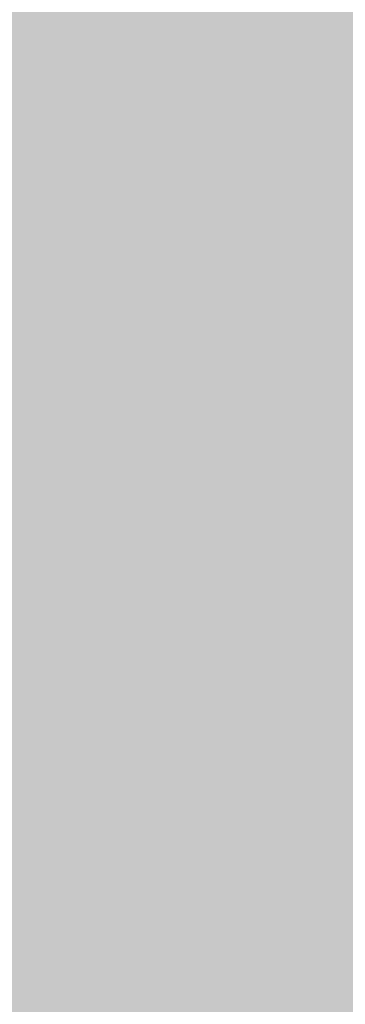
# Model space of a CAD drawing. Units: millimetres. Extents: x 0 to 2267, y 0 to 1823.
# Tile 42 of 256: x 1593.4507 to 1593.5605, y 1226.3857 to 1226.718. Entities that reach past the tile are written whole.
import ezdxf

# ---------------------------------------------------------------- set-up
doc = ezdxf.new("R2010")
doc.units = ezdxf.units.MM
doc.header["$MEASUREMENT"] = 0
doc.layers.add('M-HATC', color=252, linetype='Continuous', lineweight=18)

msp = doc.modelspace()

# ---------------------------------------------------------------- hatches: boundary and pattern name
at = {"layer": 'M-HATC'}
h = msp.add_hatch(color=256, dxfattribs=at)
h.dxf.hatch_style = 1
h.paths.add_polyline_path([(2055.77105, 1603.06204), (1381.08677, 1603.06204), (1381.08677, 1598.06204), (2055.77105, 1598.06204)])
h.paths.add_polyline_path([(2055.77105, 1598.06204), (1381.08677, 1598.06204), (1381.08677, 1593.06204), (2055.77105, 1593.06204)])
h.paths.add_polyline_path([(2051.30737, 1536.76088), (1385.55044, 1536.76088), (1385.55044, 1526.76088), (1387.55044, 1526.76088), (1388.53662, 1525.05276), (1385.33187, 1521.23348), (1385.33187, 1521.22256), (2050.25417, 1522.74913), (2048.32119, 1525.05276), (2049.30737, 1526.76088), (2051.30737, 1526.76088)])
edge = h.paths.add_edge_path()
edge.add_arc((1847.53451, 1379.14917), 135, 222.6030607, 222.8908505, ccw=False)
edge.add_line((1748.16629, 1287.76561), (1683.09212, 1287.76561))
edge.add_arc((1583.7239, 1379.14917), 135, 317.1091495, 317.3969393, ccw=False)
edge.add_arc((1678.9686, 1290.67067), 5, 222.89085, 317.10915, ccw=False)
edge.add_arc((1774.21331, 1379.14917), 135, 222.6030607, 222.8908505, ccw=False)
edge.add_line((1674.84509, 1287.76561), (1609.77092, 1287.76561))
edge.add_arc((1510.4027, 1379.14917), 135, 317.1091495, 317.3969393, ccw=False)
edge.add_arc((1605.6474, 1290.67067), 5, 222.89085, 317.10915, ccw=False)
edge.add_arc((1700.89211, 1379.14917), 135, 222.6030607, 222.8908505, ccw=False)
edge.add_line((1601.52388, 1287.76561), (1536.44972, 1287.76561))
edge.add_arc((1437.08149, 1379.14917), 135, 317.1091495, 317.3969393, ccw=False)
edge.add_arc((1532.3262, 1290.67067), 5, 222.89085, 317.10915, ccw=False)
edge.add_arc((1627.57091, 1379.14917), 135, 222.6030607, 222.8908505, ccw=False)
edge.add_line((1528.20268, 1287.76561), (1505.92891, 1287.76561))
edge.add_spline(control_points=[(1505.92891, 1287.76561), (1504.26224, 1287.76561), (1504.26224, 1282.76561), (1505.92891, 1282.76561)], knot_values=[0, 0, 0, 0, 5, 5, 5, 5], degree=3, periodic=0)
edge.add_line((1505.92891, 1282.76561), (1930.92891, 1282.76561))
edge.add_spline(control_points=[(1930.92891, 1282.76561), (1932.59557, 1282.76561), (1932.59557, 1287.76561), (1930.92891, 1287.76561)], knot_values=[0, 0, 0, 0, 5, 5, 5, 5], degree=3, periodic=0)
edge.add_line((1930.92891, 1287.76561), (1903.05573, 1287.76561))
edge.add_arc((1803.6875, 1379.14917), 135, 317.1091495, 317.3969393, ccw=False)
edge.add_arc((1898.93221, 1290.67067), 5, 222.89085, 317.10915, ccw=False)
edge.add_arc((1994.17691, 1379.14917), 135, 222.6030607, 222.8908505, ccw=False)
edge.add_line((1894.80869, 1287.76561), (1829.73452, 1287.76561))
edge.add_arc((1730.3663, 1379.14917), 135, 317.1091495, 317.3969393, ccw=False)
edge.add_arc((1825.61101, 1290.67067), 5, 222.89085, 317.10915, ccw=False)
edge.add_arc((1920.85571, 1379.14917), 135, 222.6030607, 222.8908505, ccw=False)
edge.add_line((1821.48749, 1287.76561), (1756.41332, 1287.76561))
edge.add_arc((1657.0451, 1379.14917), 135, 317.1091495, 317.3969393, ccw=False)
edge.add_arc((1752.28981, 1290.67067), 5, 222.89085, 317.10915, ccw=False)
edge = h.paths.add_edge_path()
edge.add_spline(control_points=[(1843.42891, 1227.24746), (1845.09557, 1227.24746), (1845.09557, 1232.24746), (1843.42891, 1232.24746)], knot_values=[0, 0, 0, 0, 5, 5, 5, 5], degree=3, periodic=0)
edge.add_line((1843.42891, 1232.24746), (1593.42891, 1232.24746))
edge.add_spline(control_points=[(1593.42891, 1232.24746), (1591.76224, 1232.24746), (1591.76224, 1227.24746), (1593.42891, 1227.24746)], knot_values=[0, 0, 0, 0, 5, 5, 5, 5], degree=3, periodic=0)
edge.add_line((1593.42891, 1227.24746), (1843.42891, 1227.24746))
h.paths.add_polyline_path([(1905.92891, 1127.41706), (1530.92891, 1127.41706, 0.414214), (1520.92891, 1117.41706), (1530.92891, 1117.41706), (1915.92891, 1117.41706, 0.414214)])
edge = h.paths.add_edge_path()
edge.add_arc((1397.08577, 1498.40775), 12.72993, 90.782146, 190.878706, ccw=False)
edge.add_line((1396.912, 1511.13649), (1428.00968, 1511.34875))
edge.add_line((1428.00968, 1511.34875), (1433.00968, 1511.34875))
edge.add_line((1433.00968, 1511.34875), (1434.439, 1511.34875))
edge.add_arc((1419.474, 1498.08041), 20, 41.560995, 74.082109)
edge.add_line((1424.95919, 1517.31353), (1399.93509, 1517.25608))
edge.add_spline(control_points=[(1399.93074, 1517.25607), (1399.88398, 1517.21312), (1399.8328, 1517.16893), (1399.77741, 1517.1236)], knot_values=[11.567499, 11.567499, 11.567499, 11.567499, 11.814249, 11.814249, 11.814249, 11.814249], degree=3, periodic=0)
edge.add_spline(control_points=[(1399.63279, 1517.00986), (1399.58305, 1516.97214), (1399.53072, 1516.93375), (1399.47591, 1516.89474)], knot_values=[11.167718, 11.167718, 11.167718, 11.167718, 11.365188, 11.365188, 11.365188, 11.365188], degree=3, periodic=0)
edge.add_spline(control_points=[(1399.33981, 1516.80007), (1399.15144, 1516.67185), (1398.93836, 1516.5377), (1398.70404, 1516.39942)], knot_values=[10.376405, 10.376405, 10.376405, 10.376405, 11.00994, 11.00994, 11.00994, 11.00994], degree=3, periodic=0)
edge.add_spline(control_points=[(1398.65716, 1516.37187), (1398.57885, 1516.32602), (1398.49825, 1516.27974), (1398.41549, 1516.23309)], knot_values=[10.125175, 10.125175, 10.125175, 10.125175, 10.334406, 10.334406, 10.334406, 10.334406], degree=3, periodic=0)
edge.add_spline(control_points=[(1398.26422, 1516.14874), (1398.19595, 1516.11107), (1398.12634, 1516.07319), (1398.05546, 1516.03513)], knot_values=[9.832246, 9.832246, 9.832246, 9.832246, 9.999658, 9.999658, 9.999658, 9.999658], degree=3, periodic=0)
edge.add_spline(control_points=[(1397.9987, 1516.00476), (1397.73115, 1515.86211), (1397.44602, 1515.71707), (1397.14664, 1515.57138)], knot_values=[9.161808, 9.161808, 9.161808, 9.161808, 9.787769, 9.787769, 9.787769, 9.787769], degree=3, periodic=0)
edge.add_spline(control_points=[(1397.14664, 1515.57138), (1396.84182, 1515.42305), (1396.52223, 1515.27404), (1396.1914, 1515.12621)], knot_values=[8.524455, 8.524455, 8.524455, 8.524455, 9.161808, 9.161808, 9.161808, 9.161808], degree=3, periodic=0)
edge.add_spline(control_points=[(1396.07771, 1515.07565), (1395.98538, 1515.03478), (1395.89222, 1514.99402), (1395.7983, 1514.9534)], knot_values=[8.275193, 8.275193, 8.275193, 8.275193, 8.451726, 8.451726, 8.451726, 8.451726], degree=3, periodic=0)
edge.add_spline(control_points=[(1395.60184, 1514.86912), (1395.49975, 1514.82568), (1395.39685, 1514.78244), (1395.29322, 1514.73944)], knot_values=[7.962917, 7.962917, 7.962917, 7.962917, 8.152764, 8.152764, 8.152764, 8.152764], degree=3, periodic=0)
edge.add_spline(control_points=[(1395.21158, 1514.70568), (1394.82779, 1514.5475), (1394.43452, 1514.39287), (1394.03645, 1514.24422)], knot_values=[7.21254, 7.21254, 7.21254, 7.21254, 7.913148, 7.913148, 7.913148, 7.913148], degree=3, periodic=0)
edge.add_spline(control_points=[(1394.03645, 1514.24422), (1393.70758, 1514.12142), (1393.37544, 1514.0027), (1393.04267, 1513.88945)], knot_values=[6.633733, 6.633733, 6.633733, 6.633733, 7.21254, 7.21254, 7.21254, 7.21254], degree=3, periodic=0)
edge.add_spline(control_points=[(1392.82142, 1513.81499), (1392.71978, 1513.78118), (1392.61815, 1513.74791), (1392.51658, 1513.71521)], knot_values=[6.328796, 6.328796, 6.328796, 6.328796, 6.505493, 6.505493, 6.505493, 6.505493], degree=3, periodic=0)
edge.add_spline(control_points=[(1392.51658, 1513.71521), (1392.31873, 1513.65151), (1392.12116, 1513.59001), (1391.92441, 1513.53098)], knot_values=[5.984605, 5.984605, 5.984605, 5.984605, 6.328796, 6.328796, 6.328796, 6.328796], degree=3, periodic=0)
edge.add_spline(control_points=[(1391.79155, 1513.49146), (1391.31215, 1513.35011), (1390.83842, 1513.22392), (1390.37844, 1513.11711)], knot_values=[5.066697, 5.066697, 5.066697, 5.066697, 5.907055, 5.907055, 5.907055, 5.907055], degree=3, periodic=0)
edge.add_spline(control_points=[(1390.37844, 1513.11711), (1390.17973, 1513.07097), (1389.98359, 1513.02845), (1389.79067, 1512.98988)], knot_values=[4.70367, 4.70367, 4.70367, 4.70367, 5.066695, 5.066695, 5.066695, 5.066695], degree=3, periodic=0)
edge.add_spline(control_points=[(1389.42203, 1512.92036), (1389.24588, 1512.88922), (1389.0729, 1512.86172), (1388.90364, 1512.83814)], knot_values=[4.130571, 4.130571, 4.130571, 4.130571, 4.469816, 4.469816, 4.469816, 4.469816], degree=3, periodic=0)
edge.add_spline(control_points=[(1388.90364, 1512.83814), (1388.59103, 1512.7946), (1388.29108, 1512.76444), (1388.00714, 1512.74941)], knot_values=[3.504031, 3.504031, 3.504031, 3.504031, 4.130571, 4.130571, 4.130571, 4.130571], degree=3, periodic=0)
edge.add_spline(control_points=[(1387.9356, 1512.74593), (1387.85378, 1512.74231), (1387.77334, 1512.73997), (1387.69435, 1512.73898)], knot_values=[3.268866, 3.268866, 3.268866, 3.268866, 3.451164, 3.451164, 3.451164, 3.451164], degree=3, periodic=0)
edge.add_spline(control_points=[(1387.33512, 1512.74426), (1387.20757, 1512.74991), (1387.08472, 1512.7597), (1386.96699, 1512.77385)], knot_values=[2.670686, 2.670686, 2.670686, 2.670686, 2.984, 2.984, 2.984, 2.984], degree=3, periodic=0)
edge.add_spline(control_points=[(1386.83274, 1512.79225), (1386.82093, 1512.79407), (1386.80917, 1512.79594), (1386.79747, 1512.79787)], knot_values=[2.516981, 2.516981, 2.516981, 2.516981, 2.549528, 2.549528, 2.549528, 2.549528], degree=3, periodic=0)
edge.add_spline(control_points=[(1386.45257, 1512.87348), (1386.42573, 1512.88105), (1386.39931, 1512.88895), (1386.3733, 1512.89719)], knot_values=[2.095869, 2.095869, 2.095869, 2.095869, 2.17941, 2.17941, 2.17941, 2.17941], degree=3, periodic=0)
edge.add_spline(control_points=[(1386.06911, 1513.01889), (1386.06338, 1513.02174), (1386.05768, 1513.02463), (1386.05201, 1513.02753)], knot_values=[1.72453, 1.72453, 1.72453, 1.72453, 1.745933, 1.745933, 1.745933, 1.745933], degree=3, periodic=0)
edge.add_arc((1399.474, 1498.08041), 20, 131.824322, 180)
edge.add_arc((1630.33362, 1505.54843), 250.97076, 181.7051759, 236.427975)
edge.add_arc((1605.33992, 1483.30441), 218.7822, 238.660829, 243.3496099)
edge.add_arc((1647.09105, 1510.35917), 262.89859, 183.1298361, 237.8534422, ccw=False)
h.paths.add_polyline_path([(1406.53685, 1391.96444, 0.149382), (1491.55061, 1296.44177, -0.129517)], flags=17)
edge = h.paths.add_edge_path()
edge.add_arc((2037.38381, 1498.08041), 20, 0, 48.265868)
edge.add_spline(control_points=[(2050.69731, 1513.00525), (2050.65121, 1512.98471), (2050.60338, 1512.96554), (2050.55388, 1512.94771)], knot_values=[1.835652, 1.835652, 1.835652, 1.835652, 2.000781, 2.000781, 2.000781, 2.000781], degree=3, periodic=0)
edge.add_spline(control_points=[(2050.46156, 1512.91661), (2050.479, 1512.9221), (2050.49625, 1512.92774), (2050.51332, 1512.93353)], knot_values=[2.045477, 2.045477, 2.045477, 2.045477, 2.101389, 2.101389, 2.101389, 2.101389], degree=3, periodic=0)
edge.add_spline(control_points=[(2050.12896, 1512.83416), (2050.19843, 1512.84734), (2050.26573, 1512.86233), (2050.33075, 1512.87919)], knot_values=[2.237629, 2.237629, 2.237629, 2.237629, 2.435841, 2.435841, 2.435841, 2.435841], degree=3, periodic=0)
edge.add_spline(control_points=[(2050.09463, 1512.82783), (2050.10613, 1512.82989), (2050.11757, 1512.832), (2050.12896, 1512.83416)], knot_values=[2.435841, 2.435841, 2.435841, 2.435841, 2.468321, 2.468321, 2.468321, 2.468321], degree=3, periodic=0)
edge.add_spline(control_points=[(2049.78433, 1512.78511), (2049.85521, 1512.79219), (2049.92435, 1512.80077), (2049.99166, 1512.81088)], knot_values=[2.563852, 2.563852, 2.563852, 2.563852, 2.748541, 2.748541, 2.748541, 2.748541], degree=3, periodic=0)
edge.add_spline(control_points=[(2049.4052, 1512.76169), (2049.5364, 1512.76526), (2049.66292, 1512.77299), (2049.78433, 1512.78511)], knot_values=[2.748541, 2.748541, 2.748541, 2.748541, 3.064882, 3.064882, 3.064882, 3.064882], degree=3, periodic=0)
edge.add_spline(control_points=[(2049.16976, 1512.75968), (2049.23364, 1512.7591), (2049.29654, 1512.7594), (2049.35844, 1512.7606)], knot_values=[3.102309, 3.102309, 3.102309, 3.102309, 3.2503, 3.2503, 3.2503, 3.2503], degree=3, periodic=0)
edge.add_spline(control_points=[(2048.85727, 1512.76911), (2048.96378, 1512.76378), (2049.068, 1512.76061), (2049.16976, 1512.75968)], knot_values=[3.2503, 3.2503, 3.2503, 3.2503, 3.486069, 3.486069, 3.486069, 3.486069], degree=3, periodic=0)
edge.add_spline(control_points=[(2048.69241, 1512.77892), (2048.3729, 1512.80093), (2048.0345, 1512.84106), (2047.68175, 1512.89697)], knot_values=[3.606429, 3.606429, 3.606429, 3.606429, 4.2989, 4.2989, 4.2989, 4.2989], degree=3, periodic=0)
edge.add_spline(control_points=[(2047.68175, 1512.89697), (2047.5458, 1512.91852), (2047.40772, 1512.94241), (2047.26776, 1512.96851)], knot_values=[4.2989, 4.2989, 4.2989, 4.2989, 4.565769, 4.565769, 4.565769, 4.565769], degree=3, periodic=0)
edge.add_spline(control_points=[(2047.26776, 1512.96851), (2047.14494, 1512.99141), (2047.02067, 1513.01601), (2046.89514, 1513.04223)], knot_values=[4.565769, 4.565769, 4.565769, 4.565769, 4.799971, 4.799971, 4.799971, 4.799971], degree=3, periodic=0)
edge.add_spline(control_points=[(2046.89514, 1513.04223), (2046.52865, 1513.11875), (2046.15135, 1513.20899), (2045.7676, 1513.31068)], knot_values=[4.799971, 4.799971, 4.799971, 4.799971, 5.483718, 5.483718, 5.483718, 5.483718], degree=3, periodic=0)
edge.add_spline(control_points=[(2045.7676, 1513.31068), (2045.3724, 1513.41539), (2044.97036, 1513.53225), (2044.56625, 1513.65876)], knot_values=[5.483718, 5.483718, 5.483718, 5.483718, 6.187866, 6.187866, 6.187866, 6.187866], degree=3, periodic=0)
edge.add_spline(control_points=[(2044.56625, 1513.65876), (2044.41491, 1513.70614), (2044.26329, 1513.75487), (2044.11163, 1513.80482)], knot_values=[6.187866, 6.187866, 6.187866, 6.187866, 6.451551, 6.451551, 6.451551, 6.451551], degree=3, periodic=0)
edge.add_spline(control_points=[(2044.11163, 1513.80482), (2043.99666, 1513.84269), (2043.88167, 1513.88126), (2043.76676, 1513.92048)], knot_values=[6.451551, 6.451551, 6.451551, 6.451551, 6.651434, 6.651434, 6.651434, 6.651434], degree=3, periodic=0)
edge.add_spline(control_points=[(2043.76676, 1513.92048), (2043.37157, 1514.05536), (2042.97738, 1514.19789), (2042.58863, 1514.34575)], knot_values=[6.651434, 6.651434, 6.651434, 6.651434, 7.338879, 7.338879, 7.338879, 7.338879], degree=3, periodic=0)
edge.add_spline(control_points=[(2042.58863, 1514.34575), (2042.16431, 1514.50715), (2041.74647, 1514.67491), (2041.34086, 1514.84603)], knot_values=[7.338879, 7.338879, 7.338879, 7.338879, 8.089209, 8.089209, 8.089209, 8.089209], degree=3, periodic=0)
edge.add_spline(control_points=[(2041.34086, 1514.84603), (2041.1028, 1514.94647), (2040.86896, 1515.04806), (2040.64049, 1515.1502)], knot_values=[8.089209, 8.089209, 8.089209, 8.089209, 8.529587, 8.529587, 8.529587, 8.529587], degree=3, periodic=0)
edge.add_spline(control_points=[(2040.50999, 1515.20887), (2040.08238, 1515.40218), (2039.67475, 1515.59705), (2039.29495, 1515.78939)], knot_values=[8.613818, 8.613818, 8.613818, 8.613818, 9.44571, 9.44571, 9.44571, 9.44571], degree=3, periodic=0)
edge.add_spline(control_points=[(2039.29495, 1515.78939), (2039.0618, 1515.90746), (2038.83914, 1516.02458), (2038.62878, 1516.1398)], knot_values=[9.44571, 9.44571, 9.44571, 9.44571, 9.956404, 9.956404, 9.956404, 9.956404], degree=3, periodic=0)
edge.add_spline(control_points=[(2038.62878, 1516.1398), (2038.51874, 1516.20007), (2038.41207, 1516.25982), (2038.30903, 1516.31891)], knot_values=[9.956404, 9.956404, 9.956404, 9.956404, 10.223542, 10.223542, 10.223542, 10.223542], degree=3, periodic=0)
edge.add_spline(control_points=[(2038.30903, 1516.31891), (2038.21377, 1516.37354), (2038.12161, 1516.42762), (2038.03275, 1516.48102)], knot_values=[10.223542, 10.223542, 10.223542, 10.223542, 10.47051, 10.47051, 10.47051, 10.47051], degree=3, periodic=0)
edge.add_spline(control_points=[(2038.03275, 1516.48102), (2037.78552, 1516.62961), (2037.56388, 1516.77304), (2037.37225, 1516.909)], knot_values=[10.47051, 10.47051, 10.47051, 10.47051, 11.15767, 11.15767, 11.15767, 11.15767], degree=3, periodic=0)
edge.add_spline(control_points=[(2037.37225, 1516.909), (2037.27893, 1516.9752), (2037.19274, 1517.03963), (2037.11417, 1517.10203)], knot_values=[11.15767, 11.15767, 11.15767, 11.15767, 11.49227, 11.49227, 11.49227, 11.49227], degree=3, periodic=0)
edge.add_spline(control_points=[(2036.85638, 1517.32585), (2036.91481, 1517.26923), (2036.98143, 1517.21027), (2037.05573, 1517.14922)], knot_values=[11.577341, 11.577341, 11.577341, 11.577341, 11.91035, 11.91035, 11.91035, 11.91035], degree=3, periodic=0)
edge.add_spline(control_points=[(2036.80739, 1517.37475), (2036.82301, 1517.35865), (2036.83935, 1517.34235), (2036.85638, 1517.32585)], knot_values=[11.91035, 11.91035, 11.91035, 11.91035, 12.007402, 12.007402, 12.007402, 12.007402], degree=3, periodic=0)
edge.add_spline(control_points=[(2036.70167, 1517.494), (2036.71042, 1517.48299), (2036.71958, 1517.47185), (2036.72913, 1517.4606)], knot_values=[12.184155, 12.184155, 12.184155, 12.184155, 12.255409, 12.255409, 12.255409, 12.255409], degree=3, periodic=0)
edge.add_spline(control_points=[(2036.6159, 1517.6205), (2036.61998, 1517.61304), (2036.6243, 1517.6055), (2036.62885, 1517.59789)], knot_values=[12.487913, 12.487913, 12.487913, 12.487913, 12.541035, 12.541035, 12.541035, 12.541035], degree=3, periodic=0)
edge.add_spline(control_points=[(2036.56349, 1517.78599), (2036.56372, 1517.77936), (2036.56423, 1517.77264), (2036.56502, 1517.76582)], knot_values=[12.911761, 12.911761, 12.911761, 12.911761, 12.968286, 12.968286, 12.968286, 12.968286], degree=3, periodic=0)
edge.add_spline(control_points=[(2036.61663, 1517.93042), (2036.61248, 1517.92586), (2036.60857, 1517.92121), (2036.60491, 1517.91648)], knot_values=[13.382527, 13.382527, 13.382527, 13.382527, 13.433791, 13.433791, 13.433791, 13.433791], degree=3, periodic=0)
edge.add_spline(control_points=[(2036.74902, 1518.01695), (2036.73613, 1518.0116), (2036.72393, 1518.00601), (2036.71242, 1518.00018)], knot_values=[13.726299, 13.726299, 13.726299, 13.726299, 13.809928, 13.809928, 13.809928, 13.809928], degree=3, periodic=0)
edge.add_spline(control_points=[(2036.86043, 1518.05285), (2036.83863, 1518.04743), (2036.81809, 1518.04156), (2036.79879, 1518.03526)], knot_values=[13.910887, 13.910887, 13.910887, 13.910887, 14.02153, 14.02153, 14.02153, 14.02153], degree=3, periodic=0)
edge.add_line((2036.96387, 1518.08041), (2032.38381, 1518.08041))
edge.add_line((2032.38381, 1518.08041), (2027.38381, 1518.08041))
edge.add_line((2027.38381, 1518.08041), (2022.38381, 1518.08041))
edge.add_line((2022.38381, 1518.08041), (2017.38381, 1518.08041))
edge.add_arc((2017.38381, 1498.08041), 20, 90, 138.439005)
edge.add_line((2002.41881, 1511.34875), (2003.84813, 1511.34875))
edge.add_line((2003.84813, 1511.34875), (2008.84813, 1511.34875))
edge.add_line((2008.84813, 1511.34875), (2039.77204, 1511.13768))
edge.add_arc((2039.77204, 1498.40775), 12.72993, -10.878706, 90, ccw=False)
edge.add_arc((1789.76676, 1510.35917), 262.89859, 302.1465578, 356.8701639, ccw=False)
edge.add_arc((1831.51789, 1483.30441), 218.7822, 296.6503901, 301.339171)
edge.add_arc((1806.52419, 1505.54843), 250.97076, 303.572025, 358.2948241)
h.paths.add_polyline_path([(2030.32096, 1391.96444, -0.129517), (1945.3072, 1296.44177, 0.149382)], flags=17)
edge = h.paths.add_edge_path()
edge.add_spline(control_points=[(2037.2464, 1518.08209), (2037.28977, 1518.08098), (2037.33555, 1518.08041), (2037.3838, 1518.08041)], knot_values=[0.000012, 0.000012, 0.000012, 0.000012, 0.144754, 0.144754, 0.144754, 0.144754], degree=3, periodic=0)
edge.add_line((2037.33571, 1518.08041), (2037.00963, 1518.08041))
edge.add_spline(control_points=[(2037.00963, 1518.08041), (2036.98217, 1518.07678), (2036.95605, 1518.07266), (2036.93124, 1518.06808)], knot_values=[14.13465, 14.13465, 14.13465, 14.13465, 14.247197, 14.247197, 14.247197, 14.247197], degree=3, periodic=0)
edge.add_spline(control_points=[(2036.93124, 1518.06808), (2036.92764, 1518.06741), (2036.92407, 1518.06674), (2036.92053, 1518.06605)], knot_values=[14.118315, 14.118315, 14.118315, 14.118315, 14.13465, 14.13465, 14.13465, 14.13465], degree=3, periodic=0)
edge.add_spline(control_points=[(2036.92053, 1518.06605), (2036.9118, 1518.06436), (2036.90323, 1518.06262), (2036.89484, 1518.06081)], knot_values=[14.078086, 14.078086, 14.078086, 14.078086, 14.118315, 14.118315, 14.118315, 14.118315], degree=3, periodic=0)
edge.add_spline(control_points=[(2036.89484, 1518.06081), (2036.88304, 1518.05827), (2036.87157, 1518.05562), (2036.86043, 1518.05285)], knot_values=[14.02153, 14.02153, 14.02153, 14.02153, 14.078086, 14.078086, 14.078086, 14.078086], degree=3, periodic=0)
edge.add_spline(control_points=[(2036.86043, 1518.05285), (2036.83863, 1518.04743), (2036.81809, 1518.04156), (2036.79879, 1518.03526)], knot_values=[13.910887, 13.910887, 13.910887, 13.910887, 14.02153, 14.02153, 14.02153, 14.02153], degree=3, periodic=0)
edge.add_spline(control_points=[(2036.79879, 1518.03526), (2036.79809, 1518.03504), (2036.7974, 1518.03481), (2036.79671, 1518.03458)], knot_values=[13.906906, 13.906906, 13.906906, 13.906906, 13.910887, 13.910887, 13.910887, 13.910887], degree=3, periodic=0)
edge.add_spline(control_points=[(2036.79671, 1518.03458), (2036.78819, 1518.03178), (2036.77991, 1518.02888), (2036.77187, 1518.02591)], knot_values=[13.857826, 13.857826, 13.857826, 13.857826, 13.906906, 13.906906, 13.906906, 13.906906], degree=3, periodic=0)
edge.add_spline(control_points=[(2036.77187, 1518.02591), (2036.76402, 1518.023), (2036.75641, 1518.02002), (2036.74902, 1518.01695)], knot_values=[13.809928, 13.809928, 13.809928, 13.809928, 13.857826, 13.857826, 13.857826, 13.857826], degree=3, periodic=0)
edge.add_spline(control_points=[(2036.74902, 1518.01695), (2036.73613, 1518.0116), (2036.72393, 1518.00601), (2036.71242, 1518.00018)], knot_values=[13.726299, 13.726299, 13.726299, 13.726299, 13.809928, 13.809928, 13.809928, 13.809928], degree=3, periodic=0)
edge.add_spline(control_points=[(2036.71242, 1518.00018), (2036.71211, 1518.00002), (2036.71179, 1517.99986), (2036.71147, 1517.99969)], knot_values=[13.723993, 13.723993, 13.723993, 13.723993, 13.726299, 13.726299, 13.726299, 13.726299], degree=3, periodic=0)
edge.add_spline(control_points=[(2036.71147, 1517.99969), (2036.70634, 1517.99708), (2036.70134, 1517.99441), (2036.69648, 1517.9917)], knot_values=[13.686536, 13.686536, 13.686536, 13.686536, 13.723993, 13.723993, 13.723993, 13.723993], degree=3, periodic=0)
edge.add_spline(control_points=[(2036.69648, 1517.9917), (2036.6919, 1517.98914), (2036.68744, 1517.98654), (2036.6831, 1517.9839)], knot_values=[13.651251, 13.651251, 13.651251, 13.651251, 13.686536, 13.686536, 13.686536, 13.686536], degree=3, periodic=0)
edge.add_spline(control_points=[(2036.6831, 1517.9839), (2036.67641, 1517.97983), (2036.67001, 1517.97566), (2036.6639, 1517.97139)], knot_values=[13.596804, 13.596804, 13.596804, 13.596804, 13.651251, 13.651251, 13.651251, 13.651251], degree=3, periodic=0)
edge.add_spline(control_points=[(2036.6639, 1517.97139), (2036.66358, 1517.97117), (2036.66326, 1517.97094), (2036.66294, 1517.97072)], knot_values=[13.593956, 13.593956, 13.593956, 13.593956, 13.596804, 13.596804, 13.596804, 13.596804], degree=3, periodic=0)
edge.add_spline(control_points=[(2036.66294, 1517.97072), (2036.6603, 1517.96886), (2036.65771, 1517.96698), (2036.65518, 1517.96509)], knot_values=[13.570322, 13.570322, 13.570322, 13.570322, 13.593956, 13.593956, 13.593956, 13.593956], degree=3, periodic=0)
edge.add_spline(control_points=[(2036.65518, 1517.96509), (2036.65251, 1517.9631), (2036.64991, 1517.96108), (2036.64737, 1517.95905)], knot_values=[13.545477, 13.545477, 13.545477, 13.545477, 13.570322, 13.570322, 13.570322, 13.570322], degree=3, periodic=0)
edge.add_spline(control_points=[(2036.64737, 1517.95905), (2036.64721, 1517.95892), (2036.64705, 1517.9588), (2036.64689, 1517.95867)], knot_values=[13.543931, 13.543931, 13.543931, 13.543931, 13.545477, 13.545477, 13.545477, 13.545477], degree=3, periodic=0)
edge.add_spline(control_points=[(2036.64689, 1517.95867), (2036.64121, 1517.95411), (2036.63582, 1517.94945), (2036.63073, 1517.94468)], knot_values=[13.488237, 13.488237, 13.488237, 13.488237, 13.543931, 13.543931, 13.543931, 13.543931], degree=3, periodic=0)
edge.add_spline(control_points=[(2036.63073, 1517.94468), (2036.62817, 1517.94229), (2036.62569, 1517.93988), (2036.62329, 1517.93744)], knot_values=[13.460307, 13.460307, 13.460307, 13.460307, 13.488237, 13.488237, 13.488237, 13.488237], degree=3, periodic=0)
edge.add_spline(control_points=[(2036.62329, 1517.93744), (2036.62151, 1517.93564), (2036.61978, 1517.93383), (2036.61809, 1517.932)], knot_values=[13.439712, 13.439712, 13.439712, 13.439712, 13.460307, 13.460307, 13.460307, 13.460307], degree=3, periodic=0)
edge.add_spline(control_points=[(2036.61809, 1517.932), (2036.6176, 1517.93147), (2036.61711, 1517.93095), (2036.61663, 1517.93042)], knot_values=[13.433791, 13.433791, 13.433791, 13.433791, 13.439712, 13.439712, 13.439712, 13.439712], degree=3, periodic=0)
edge.add_spline(control_points=[(2036.61663, 1517.93042), (2036.61248, 1517.92586), (2036.60857, 1517.92121), (2036.60491, 1517.91648)], knot_values=[13.382527, 13.382527, 13.382527, 13.382527, 13.433791, 13.433791, 13.433791, 13.433791], degree=3, periodic=0)
edge.add_spline(control_points=[(2036.60491, 1517.91648), (2036.60258, 1517.91347), (2036.60036, 1517.91044), (2036.59824, 1517.90737)], knot_values=[13.350017, 13.350017, 13.350017, 13.350017, 13.382527, 13.382527, 13.382527, 13.382527], degree=3, periodic=0)
edge.add_spline(control_points=[(2036.59824, 1517.90737), (2036.59718, 1517.90585), (2036.59616, 1517.90433), (2036.59515, 1517.90279)], knot_values=[13.333922, 13.333922, 13.333922, 13.333922, 13.350017, 13.350017, 13.350017, 13.350017], degree=3, periodic=0)
edge.add_spline(control_points=[(2036.59515, 1517.90279), (2036.59452, 1517.90183), (2036.5939, 1517.90086), (2036.59329, 1517.89989)], knot_values=[13.323828, 13.323828, 13.323828, 13.323828, 13.333922, 13.333922, 13.333922, 13.333922], degree=3, periodic=0)
edge.add_spline(control_points=[(2036.59329, 1517.89989), (2036.59049, 1517.89545), (2036.5879, 1517.89094), (2036.5855, 1517.88637)], knot_values=[13.277545, 13.277545, 13.277545, 13.277545, 13.323828, 13.323828, 13.323828, 13.323828], degree=3, periodic=0)
edge.add_spline(control_points=[(2036.5855, 1517.88637), (2036.58355, 1517.88267), (2036.58174, 1517.87892), (2036.58006, 1517.87513)], knot_values=[13.240119, 13.240119, 13.240119, 13.240119, 13.277545, 13.277545, 13.277545, 13.277545], degree=3, periodic=0)
edge.add_spline(control_points=[(2036.58006, 1517.87513), (2036.57952, 1517.87393), (2036.579, 1517.87272), (2036.57849, 1517.87151)], knot_values=[13.228211, 13.228211, 13.228211, 13.228211, 13.240119, 13.240119, 13.240119, 13.240119], degree=3, periodic=0)
edge.add_spline(control_points=[(2036.57849, 1517.87151), (2036.57796, 1517.87023), (2036.57744, 1517.86896), (2036.57693, 1517.86767)], knot_values=[13.215717, 13.215717, 13.215717, 13.215717, 13.228211, 13.228211, 13.228211, 13.228211], degree=3, periodic=0)
edge.add_spline(control_points=[(2036.57693, 1517.86767), (2036.57548, 1517.86399), (2036.57414, 1517.86027), (2036.57293, 1517.85651)], knot_values=[13.179847, 13.179847, 13.179847, 13.179847, 13.215717, 13.215717, 13.215717, 13.215717], degree=3, periodic=0)
edge.add_spline(control_points=[(2036.57293, 1517.85651), (2036.5713, 1517.8515), (2036.56989, 1517.84641), (2036.56868, 1517.84126)], knot_values=[13.132017, 13.132017, 13.132017, 13.132017, 13.179847, 13.179847, 13.179847, 13.179847], degree=3, periodic=0)
edge.add_spline(control_points=[(2036.56868, 1517.84126), (2036.56844, 1517.84023), (2036.56821, 1517.8392), (2036.56798, 1517.83817)], knot_values=[13.122482, 13.122482, 13.122482, 13.122482, 13.132017, 13.132017, 13.132017, 13.132017], degree=3, periodic=0)
edge.add_spline(control_points=[(2036.56798, 1517.83817), (2036.56758, 1517.83634), (2036.56721, 1517.8345), (2036.56687, 1517.83266)], knot_values=[13.105592, 13.105592, 13.105592, 13.105592, 13.122482, 13.122482, 13.122482, 13.122482], degree=3, periodic=0)
edge.add_spline(control_points=[(2036.56687, 1517.83266), (2036.56622, 1517.82921), (2036.56567, 1517.82574), (2036.5652, 1517.82223)], knot_values=[13.074063, 13.074063, 13.074063, 13.074063, 13.105592, 13.105592, 13.105592, 13.105592], degree=3, periodic=0)
edge.add_spline(control_points=[(2036.5652, 1517.82223), (2036.5652, 1517.82223), (2036.5652, 1517.82223), (2036.5652, 1517.82223)], knot_values=[13.074043, 13.074043, 13.074043, 13.074043, 13.074063, 13.074063, 13.074063, 13.074063], degree=3, periodic=0)
edge.add_spline(control_points=[(2036.5652, 1517.82223), (2036.56443, 1517.81643), (2036.5639, 1517.81055), (2036.56361, 1517.8046)], knot_values=[13.021884, 13.021884, 13.021884, 13.021884, 13.074043, 13.074043, 13.074043, 13.074043], degree=3, periodic=0)
edge.add_spline(control_points=[(2036.56361, 1517.8046), (2036.56358, 1517.80401), (2036.56356, 1517.80342), (2036.56353, 1517.80283)], knot_values=[13.01674, 13.01674, 13.01674, 13.01674, 13.021884, 13.021884, 13.021884, 13.021884], degree=3, periodic=0)
edge.add_spline(control_points=[(2036.56353, 1517.80283), (2036.56344, 1517.80051), (2036.56338, 1517.79817), (2036.56336, 1517.79582)], knot_values=[12.996438, 12.996438, 12.996438, 12.996438, 13.01674, 13.01674, 13.01674, 13.01674], degree=3, periodic=0)
edge.add_spline(control_points=[(2036.56336, 1517.79582), (2036.56334, 1517.79257), (2036.56338, 1517.78929), (2036.56349, 1517.78599)], knot_values=[12.968286, 12.968286, 12.968286, 12.968286, 12.996438, 12.996438, 12.996438, 12.996438], degree=3, periodic=0)
edge.add_spline(control_points=[(2036.56349, 1517.78599), (2036.56372, 1517.77936), (2036.56423, 1517.77264), (2036.56502, 1517.76582)], knot_values=[12.911761, 12.911761, 12.911761, 12.911761, 12.968286, 12.968286, 12.968286, 12.968286], degree=3, periodic=0)
edge.add_spline(control_points=[(2036.56502, 1517.76582), (2036.56503, 1517.76573), (2036.56504, 1517.76564), (2036.56505, 1517.76555)], knot_values=[12.911017, 12.911017, 12.911017, 12.911017, 12.911761, 12.911761, 12.911761, 12.911761], degree=3, periodic=0)
edge.add_spline(control_points=[(2036.56505, 1517.76555), (2036.56541, 1517.76245), (2036.56583, 1517.75933), (2036.56631, 1517.75619)], knot_values=[12.88528, 12.88528, 12.88528, 12.88528, 12.911017, 12.911017, 12.911017, 12.911017], degree=3, periodic=0)
edge.add_spline(control_points=[(2036.56631, 1517.75619), (2036.56673, 1517.75341), (2036.5672, 1517.75062), (2036.56771, 1517.74782)], knot_values=[12.862519, 12.862519, 12.862519, 12.862519, 12.88528, 12.88528, 12.88528, 12.88528], degree=3, periodic=0)
edge.add_spline(control_points=[(2036.56771, 1517.74782), (2036.56779, 1517.74737), (2036.56788, 1517.74692), (2036.56796, 1517.74647)], knot_values=[12.858885, 12.858885, 12.858885, 12.858885, 12.862519, 12.862519, 12.862519, 12.862519], degree=3, periodic=0)
edge.add_spline(control_points=[(2036.56796, 1517.74647), (2036.5692, 1517.73986), (2036.57069, 1517.73316), (2036.57243, 1517.72638)], knot_values=[12.8053, 12.8053, 12.8053, 12.8053, 12.858885, 12.858885, 12.858885, 12.858885], degree=3, periodic=0)
edge.add_spline(control_points=[(2036.57243, 1517.72638), (2036.5734, 1517.72257), (2036.57446, 1517.71874), (2036.57559, 1517.71488)], knot_values=[12.775176, 12.775176, 12.775176, 12.775176, 12.8053, 12.8053, 12.8053, 12.8053], degree=3, periodic=0)
edge.add_spline(control_points=[(2036.57559, 1517.71488), (2036.57628, 1517.71252), (2036.577, 1517.71015), (2036.57775, 1517.70778)], knot_values=[12.756759, 12.756759, 12.756759, 12.756759, 12.775176, 12.775176, 12.775176, 12.775176], degree=3, periodic=0)
edge.add_spline(control_points=[(2036.57775, 1517.70778), (2036.57808, 1517.70674), (2036.57841, 1517.7057), (2036.57875, 1517.70466)], knot_values=[12.748742, 12.748742, 12.748742, 12.748742, 12.756759, 12.756759, 12.756759, 12.756759], degree=3, periodic=0)
edge.add_spline(control_points=[(2036.57875, 1517.70466), (2036.58082, 1517.6983), (2036.58309, 1517.69187), (2036.58557, 1517.68537)], knot_values=[12.69959, 12.69959, 12.69959, 12.69959, 12.748742, 12.748742, 12.748742, 12.748742], degree=3, periodic=0)
edge.add_spline(control_points=[(2036.58557, 1517.68537), (2036.58762, 1517.68001), (2036.5898, 1517.6746), (2036.59213, 1517.66916)], knot_values=[12.659038, 12.659038, 12.659038, 12.659038, 12.69959, 12.69959, 12.69959, 12.69959], degree=3, periodic=0)
edge.add_spline(control_points=[(2036.59213, 1517.66916), (2036.59397, 1517.66482), (2036.59591, 1517.66047), (2036.59793, 1517.65608)], knot_values=[12.626806, 12.626806, 12.626806, 12.626806, 12.659038, 12.659038, 12.659038, 12.659038], degree=3, periodic=0)
edge.add_spline(control_points=[(2036.59793, 1517.65608), (2036.59839, 1517.65507), (2036.59886, 1517.65406), (2036.59934, 1517.65305)], knot_values=[12.619394, 12.619394, 12.619394, 12.619394, 12.626806, 12.626806, 12.626806, 12.626806], degree=3, periodic=0)
edge.add_spline(control_points=[(2036.59934, 1517.65305), (2036.60435, 1517.64236), (2036.60987, 1517.63151), (2036.61589, 1517.6205)], knot_values=[12.541039, 12.541039, 12.541039, 12.541039, 12.619394, 12.619394, 12.619394, 12.619394], degree=3, periodic=0)
edge.add_spline(control_points=[(2036.61589, 1517.6205), (2036.61589, 1517.6205), (2036.6159, 1517.6205), (2036.6159, 1517.6205)], knot_values=[12.541035, 12.541035, 12.541035, 12.541035, 12.541039, 12.541039, 12.541039, 12.541039], degree=3, periodic=0)
edge.add_spline(control_points=[(2036.6159, 1517.6205), (2036.61998, 1517.61304), (2036.6243, 1517.6055), (2036.62885, 1517.59789)], knot_values=[12.487913, 12.487913, 12.487913, 12.487913, 12.541035, 12.541035, 12.541035, 12.541035], degree=3, periodic=0)
edge.add_spline(control_points=[(2036.62885, 1517.59789), (2036.63261, 1517.5916), (2036.63653, 1517.58526), (2036.64061, 1517.57888)], knot_values=[12.443982, 12.443982, 12.443982, 12.443982, 12.487913, 12.487913, 12.487913, 12.487913], degree=3, periodic=0)
edge.add_spline(control_points=[(2036.64061, 1517.57888), (2036.64144, 1517.57757), (2036.64228, 1517.57626), (2036.64313, 1517.57495)], knot_values=[12.434996, 12.434996, 12.434996, 12.434996, 12.443982, 12.443982, 12.443982, 12.443982], degree=3, periodic=0)
edge.add_spline(control_points=[(2036.64313, 1517.57495), (2036.65306, 1517.55958), (2036.66389, 1517.54394), (2036.6756, 1517.52803)], knot_values=[12.329647, 12.329647, 12.329647, 12.329647, 12.434996, 12.434996, 12.434996, 12.434996], degree=3, periodic=0)
edge.add_spline(control_points=[(2036.6756, 1517.52803), (2036.68385, 1517.51682), (2036.69254, 1517.50548), (2036.70167, 1517.494)], knot_values=[12.255409, 12.255409, 12.255409, 12.255409, 12.329647, 12.329647, 12.329647, 12.329647], degree=3, periodic=0)
edge.add_spline(control_points=[(2036.70167, 1517.494), (2036.71042, 1517.48299), (2036.71958, 1517.47185), (2036.72913, 1517.4606)], knot_values=[12.184155, 12.184155, 12.184155, 12.184155, 12.255409, 12.255409, 12.255409, 12.255409], degree=3, periodic=0)
edge.add_spline(control_points=[(2036.72913, 1517.4606), (2036.74363, 1517.44352), (2036.75904, 1517.42617), (2036.77534, 1517.40855)], knot_values=[12.075961, 12.075961, 12.075961, 12.075961, 12.184155, 12.184155, 12.184155, 12.184155], degree=3, periodic=0)
edge.add_spline(control_points=[(2036.77534, 1517.40855), (2036.77631, 1517.4075), (2036.77729, 1517.40645), (2036.77827, 1517.40539)], knot_values=[12.069502, 12.069502, 12.069502, 12.069502, 12.075961, 12.075961, 12.075961, 12.075961], degree=3, periodic=0)
edge.add_spline(control_points=[(2036.77827, 1517.40539), (2036.78768, 1517.39526), (2036.79739, 1517.38505), (2036.80739, 1517.37475)], knot_values=[12.007402, 12.007402, 12.007402, 12.007402, 12.069502, 12.069502, 12.069502, 12.069502], degree=3, periodic=0)
edge.add_spline(control_points=[(2036.80739, 1517.37475), (2036.82301, 1517.35865), (2036.83935, 1517.34235), (2036.85638, 1517.32585)], knot_values=[11.91035, 11.91035, 11.91035, 11.91035, 12.007402, 12.007402, 12.007402, 12.007402], degree=3, periodic=0)
edge.add_spline(control_points=[(2036.85638, 1517.32585), (2036.91481, 1517.26923), (2036.98143, 1517.21027), (2037.05573, 1517.14922)], knot_values=[11.577341, 11.577341, 11.577341, 11.577341, 11.91035, 11.91035, 11.91035, 11.91035], degree=3, periodic=0)
edge.add_spline(control_points=[(2037.05573, 1517.14922), (2037.07471, 1517.13362), (2037.0942, 1517.11789), (2037.11417, 1517.10203)], knot_values=[11.49227, 11.49227, 11.49227, 11.49227, 11.577341, 11.577341, 11.577341, 11.577341], degree=3, periodic=0)
edge.add_spline(control_points=[(2037.11417, 1517.10203), (2037.19274, 1517.03963), (2037.27893, 1516.9752), (2037.37225, 1516.909)], knot_values=[11.15767, 11.15767, 11.15767, 11.15767, 11.49227, 11.49227, 11.49227, 11.49227], degree=3, periodic=0)
edge.add_spline(control_points=[(2037.37225, 1516.909), (2037.56388, 1516.77304), (2037.78552, 1516.62961), (2038.03275, 1516.48102)], knot_values=[10.47051, 10.47051, 10.47051, 10.47051, 11.15767, 11.15767, 11.15767, 11.15767], degree=3, periodic=0)
edge.add_spline(control_points=[(2038.03275, 1516.48102), (2038.12161, 1516.42762), (2038.21377, 1516.37354), (2038.30903, 1516.31891)], knot_values=[10.223542, 10.223542, 10.223542, 10.223542, 10.47051, 10.47051, 10.47051, 10.47051], degree=3, periodic=0)
edge.add_spline(control_points=[(2038.30903, 1516.31891), (2038.41207, 1516.25982), (2038.51874, 1516.20007), (2038.62878, 1516.1398)], knot_values=[9.956404, 9.956404, 9.956404, 9.956404, 10.223542, 10.223542, 10.223542, 10.223542], degree=3, periodic=0)
edge.add_spline(control_points=[(2038.62878, 1516.1398), (2038.83914, 1516.02458), (2039.0618, 1515.90746), (2039.29495, 1515.78939)], knot_values=[9.44571, 9.44571, 9.44571, 9.44571, 9.956404, 9.956404, 9.956404, 9.956404], degree=3, periodic=0)
edge.add_spline(control_points=[(2039.29495, 1515.78939), (2039.67475, 1515.59705), (2040.08238, 1515.40218), (2040.50999, 1515.20887)], knot_values=[8.613818, 8.613818, 8.613818, 8.613818, 9.44571, 9.44571, 9.44571, 9.44571], degree=3, periodic=0)
edge.add_spline(control_points=[(2040.50999, 1515.20887), (2040.55329, 1515.1893), (2040.59679, 1515.16974), (2040.64049, 1515.1502)], knot_values=[8.529587, 8.529587, 8.529587, 8.529587, 8.613818, 8.613818, 8.613818, 8.613818], degree=3, periodic=0)
edge.add_spline(control_points=[(2040.64049, 1515.1502), (2040.86896, 1515.04806), (2041.1028, 1514.94647), (2041.34086, 1514.84603)], knot_values=[8.089209, 8.089209, 8.089209, 8.089209, 8.529587, 8.529587, 8.529587, 8.529587], degree=3, periodic=0)
edge.add_spline(control_points=[(2041.34086, 1514.84603), (2041.74647, 1514.67491), (2042.16431, 1514.50715), (2042.58863, 1514.34575)], knot_values=[7.338879, 7.338879, 7.338879, 7.338879, 8.089209, 8.089209, 8.089209, 8.089209], degree=3, periodic=0)
edge.add_spline(control_points=[(2042.58863, 1514.34575), (2042.97738, 1514.19789), (2043.37157, 1514.05536), (2043.76676, 1513.92048)], knot_values=[6.651434, 6.651434, 6.651434, 6.651434, 7.338879, 7.338879, 7.338879, 7.338879], degree=3, periodic=0)
edge.add_spline(control_points=[(2043.76676, 1513.92048), (2043.88167, 1513.88126), (2043.99666, 1513.84269), (2044.11163, 1513.80482)], knot_values=[6.451551, 6.451551, 6.451551, 6.451551, 6.651434, 6.651434, 6.651434, 6.651434], degree=3, periodic=0)
edge.add_spline(control_points=[(2044.11163, 1513.80482), (2044.26329, 1513.75487), (2044.41491, 1513.70614), (2044.56625, 1513.65876)], knot_values=[6.187866, 6.187866, 6.187866, 6.187866, 6.451551, 6.451551, 6.451551, 6.451551], degree=3, periodic=0)
edge.add_spline(control_points=[(2044.56625, 1513.65876), (2044.97036, 1513.53225), (2045.3724, 1513.41539), (2045.7676, 1513.31068)], knot_values=[5.483718, 5.483718, 5.483718, 5.483718, 6.187866, 6.187866, 6.187866, 6.187866], degree=3, periodic=0)
edge.add_spline(control_points=[(2045.7676, 1513.31068), (2046.15135, 1513.20899), (2046.52865, 1513.11875), (2046.89514, 1513.04223)], knot_values=[4.799971, 4.799971, 4.799971, 4.799971, 5.483718, 5.483718, 5.483718, 5.483718], degree=3, periodic=0)
edge.add_spline(control_points=[(2046.89514, 1513.04223), (2047.02067, 1513.01601), (2047.14494, 1512.99141), (2047.26776, 1512.96851)], knot_values=[4.565769, 4.565769, 4.565769, 4.565769, 4.799971, 4.799971, 4.799971, 4.799971], degree=3, periodic=0)
edge.add_spline(control_points=[(2047.26776, 1512.96851), (2047.40772, 1512.94241), (2047.5458, 1512.91852), (2047.68175, 1512.89697)], knot_values=[4.2989, 4.2989, 4.2989, 4.2989, 4.565769, 4.565769, 4.565769, 4.565769], degree=3, periodic=0)
edge.add_spline(control_points=[(2047.68175, 1512.89697), (2048.0345, 1512.84106), (2048.3729, 1512.80093), (2048.69241, 1512.77892)], knot_values=[3.606429, 3.606429, 3.606429, 3.606429, 4.2989, 4.2989, 4.2989, 4.2989], degree=3, periodic=0)
edge.add_spline(control_points=[(2048.69241, 1512.77892), (2048.74794, 1512.7751), (2048.8029, 1512.77182), (2048.85727, 1512.76911)], knot_values=[3.486069, 3.486069, 3.486069, 3.486069, 3.606429, 3.606429, 3.606429, 3.606429], degree=3, periodic=0)
edge.add_spline(control_points=[(2048.85727, 1512.76911), (2048.96378, 1512.76378), (2049.068, 1512.76061), (2049.16976, 1512.75968)], knot_values=[3.2503, 3.2503, 3.2503, 3.2503, 3.486069, 3.486069, 3.486069, 3.486069], degree=3, periodic=0)
edge.add_spline(control_points=[(2049.16976, 1512.75968), (2049.23364, 1512.7591), (2049.29654, 1512.7594), (2049.35844, 1512.7606)], knot_values=[3.102309, 3.102309, 3.102309, 3.102309, 3.2503, 3.2503, 3.2503, 3.2503], degree=3, periodic=0)
edge.add_spline(control_points=[(2049.35844, 1512.7606), (2049.37409, 1512.76091), (2049.38968, 1512.76127), (2049.4052, 1512.76169)], knot_values=[3.064882, 3.064882, 3.064882, 3.064882, 3.102309, 3.102309, 3.102309, 3.102309], degree=3, periodic=0)
edge.add_spline(control_points=[(2049.4052, 1512.76169), (2049.5364, 1512.76526), (2049.66292, 1512.77299), (2049.78433, 1512.78511)], knot_values=[2.748541, 2.748541, 2.748541, 2.748541, 3.064882, 3.064882, 3.064882, 3.064882], degree=3, periodic=0)
edge.add_spline(control_points=[(2049.78433, 1512.78511), (2049.85521, 1512.79219), (2049.92435, 1512.80077), (2049.99166, 1512.81088)], knot_values=[2.563852, 2.563852, 2.563852, 2.563852, 2.748541, 2.748541, 2.748541, 2.748541], degree=3, periodic=0)
edge.add_spline(control_points=[(2049.99166, 1512.81088), (2050.02648, 1512.81612), (2050.0608, 1512.82177), (2050.09463, 1512.82783)], knot_values=[2.468321, 2.468321, 2.468321, 2.468321, 2.563852, 2.563852, 2.563852, 2.563852], degree=3, periodic=0)
edge.add_spline(control_points=[(2050.09463, 1512.82783), (2050.10613, 1512.82989), (2050.11757, 1512.832), (2050.12896, 1512.83416)], knot_values=[2.435841, 2.435841, 2.435841, 2.435841, 2.468321, 2.468321, 2.468321, 2.468321], degree=3, periodic=0)
edge.add_spline(control_points=[(2050.12896, 1512.83416), (2050.19843, 1512.84734), (2050.26573, 1512.86233), (2050.33075, 1512.87919)], knot_values=[2.237629, 2.237629, 2.237629, 2.237629, 2.435841, 2.435841, 2.435841, 2.435841], degree=3, periodic=0)
edge.add_spline(control_points=[(2050.33075, 1512.87919), (2050.37544, 1512.89077), (2050.41906, 1512.90324), (2050.46156, 1512.91661)], knot_values=[2.101389, 2.101389, 2.101389, 2.101389, 2.237629, 2.237629, 2.237629, 2.237629], degree=3, periodic=0)
edge.add_spline(control_points=[(2050.46156, 1512.91661), (2050.479, 1512.9221), (2050.49625, 1512.92774), (2050.51332, 1512.93353)], knot_values=[2.045477, 2.045477, 2.045477, 2.045477, 2.101389, 2.101389, 2.101389, 2.101389], degree=3, periodic=0)
edge.add_spline(control_points=[(2050.51332, 1512.93353), (2050.52696, 1512.93816), (2050.54048, 1512.94288), (2050.55388, 1512.94771)], knot_values=[2.000781, 2.000781, 2.000781, 2.000781, 2.045477, 2.045477, 2.045477, 2.045477], degree=3, periodic=0)
edge.add_spline(control_points=[(2050.55388, 1512.94771), (2050.60338, 1512.96554), (2050.65121, 1512.98471), (2050.69731, 1513.00525)], knot_values=[1.835652, 1.835652, 1.835652, 1.835652, 2.000781, 2.000781, 2.000781, 2.000781], degree=3, periodic=0)
edge.add_arc((2037.38381, 1498.08041), 20, 48.265868, 90.129934)
edge = h.paths.add_edge_path(flags=16)
edge.add_spline(control_points=[(1386.13885, 1512.98591), (1388.91997, 1511.73946), (1398.03873, 1515.51866), (1399.93074, 1517.25607)], knot_values=[1.831046, 1.831046, 1.831046, 1.831046, 11.814249, 11.814249, 11.814249, 11.814249], degree=3, periodic=0)
edge.add_line((1399.93074, 1517.25607), (1393.74348, 1517.24186))
edge.add_arc((1399.474, 1498.08041), 20, 106.650105, 131.817301)
h = msp.add_hatch(color=256, dxfattribs=at)
h.dxf.hatch_style = 1
h.paths.add_polyline_path([(2042.88863, 1580.17963), (2055.77105, 1593.06204), (1381.08677, 1593.06204), (1393.96918, 1580.17963), (1374.08597, 1560.29642), (2062.77184, 1560.29642)])
h.paths.add_polyline_path([(1843.42891, 1201.32971), (1843.42891, 1227.24746), (1593.42891, 1227.24746), (1593.42891, 1201.32971, -0.228274), (1574.59893, 1162.23457), (1530.92891, 1127.41706), (1905.92891, 1127.41706), (1862.25888, 1162.23457, -0.228274)])

doc.saveas('drawing.dxf')
